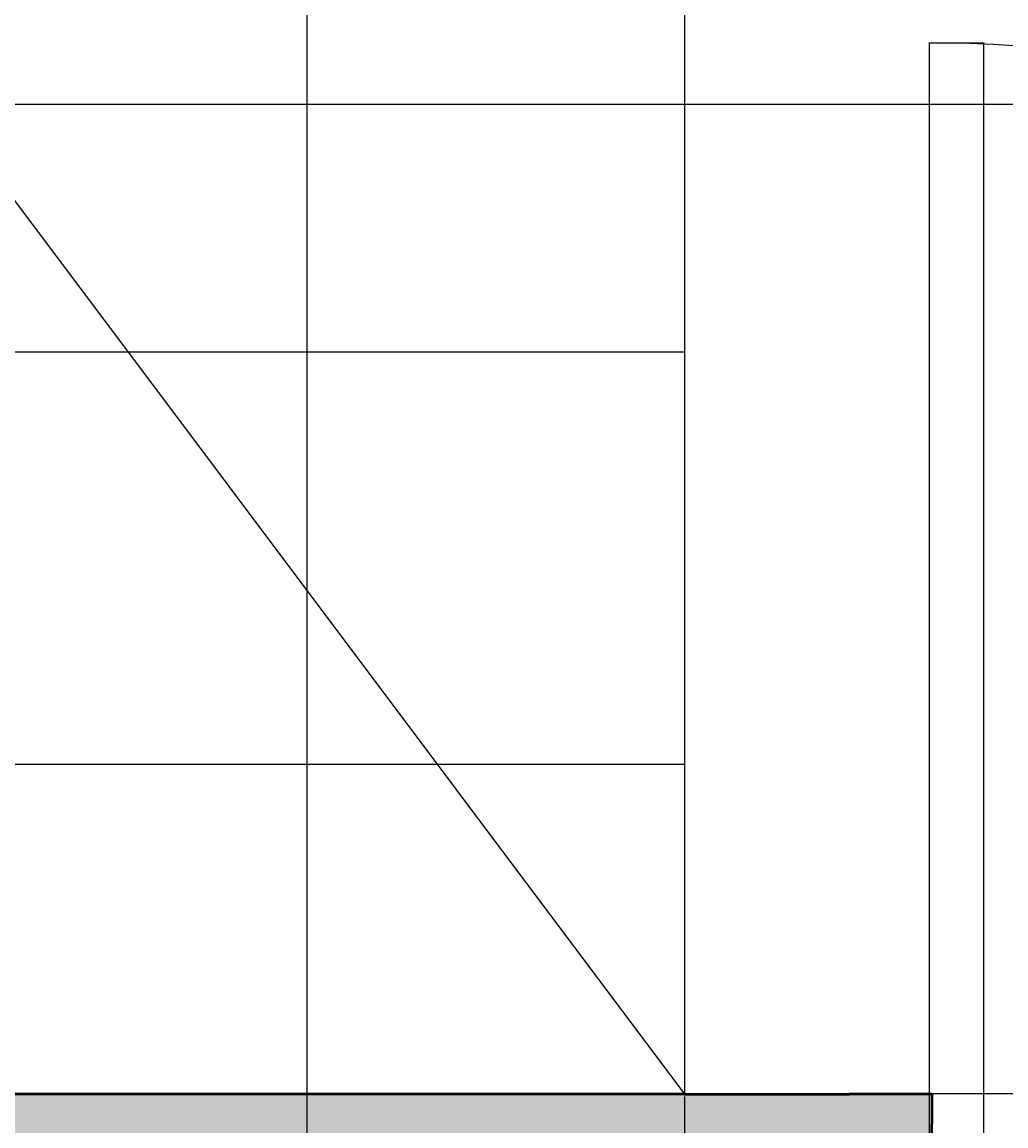
# Model space of a CAD drawing. Units: inches. Extents: x 2231 to 2461, y 2045 to 2455.
# Tile 5 of 95: x 2279 to 2303, y 2072 to 2099. Entities that reach past the tile are written whole.
import ezdxf

# ---------------------------------------------------------------- set-up
doc = ezdxf.new("R2010")
doc.units = ezdxf.units.IN
for name, color, linetype, lineweight in [('A-ANNO-DIMS', 2, 'Continuous', 18), ('A-DOOR', 3, 'Continuous', 25), ('A-FLOR-EVTR', 8, 'Continuous', 25), ('A-WALL', 7, 'Continuous', 50)]:
    doc.layers.add(name, color=color, linetype=linetype, lineweight=lineweight)
doc.layers.add('A-WALL-PATT', color=18, linetype='Continuous', lineweight=13, true_color=0x000000)
doc.styles.get("Standard").update_dxf_attribs({"font": 'arial.ttf'})
doc.dimstyles.get("Standard").update_dxf_attribs({"dimtxt": 0.18, "dimasz": 0.18, "dimexe": 0.18, "dimexo": 0.0625, "dimgap": 0.09, "dimtad": 0, "dimtih": 1, "dimtoh": 1, "dimdec": 4, "dimzin": 0, "dimdsep": 46, "dimtxsty": 'Standard', "dimcen": 0.09, "dimadec": 0, "dimazin": 0, "dimtfac": 1, "dimtdec": 4, "dimtofl": 0, "dimtmove": 0, "dimatfit": 3, "dimfxl": 1, "dimtolj": 1, "dimtzin": 0, "dimarcsym": 0})

# ---------------------------------------------------------------- blocks, each defined once
blk = doc.blocks.new('*U5')
blk.add_lwpolyline([(0, 0), (0, 40), (1.75, 40), (1.75, 0)], close=True)
blk.add_arc((0, 0), 40, 0, 90)
blk = doc.blocks.new('*D44')
at = {"layer": 'A-ANNO-DIMS', "color": 0, "lineweight": -2, "transparency": 16777216}
for p, q in [((2294.794, 2072.77), (2294.794, 2044.803)), ((2300.794, 2072.77), (2300.794, 2044.803)), ((2294.974, 2044.983), (2297.644, 2044.983)), ((2300.614, 2044.983), (2297.943, 2044.983))]:
    blk.add_line(p, q, dxfattribs=at)
at = {"layer": 'A-ANNO-DIMS', "color": 0, "transparency": 16777216}
for points in [[(2294.974, 2045.013), (2294.974, 2044.953), (2294.794, 2044.983)], [(2300.614, 2045.013), (2300.614, 2044.953), (2300.794, 2044.983)]]:
    blk.add_solid(points, dxfattribs=at)
at = {"layer": 'Defpoints', "color": 0, "transparency": 16777216}
for p in [(2294.794, 2072.833), (2300.794, 2072.833), (2300.794, 2044.983)]:
    blk.add_point(p, dxfattribs=at)
at = {"layer": 'A-ANNO-DIMS', "color": 0, "transparency": 16777216, "insert": (2297.794, 2044.983), "char_height": 0.18, "attachment_point": 5}
blk.add_mtext('\\A1;6', dxfattribs=at)
blk = doc.blocks.new('*D51')
at = {"layer": 'A-ANNO-DIMS', "color": 0, "lineweight": -2, "transparency": 16777216}
for p, q in [((2258.794, 2306.77), (2258.794, 2044.803)), ((2330.794, 2306.77), (2330.794, 2044.803)), ((2258.974, 2044.983), (2294.576, 2044.983)), ((2330.614, 2044.983), (2295.011, 2044.983))]:
    blk.add_line(p, q, dxfattribs=at)
at = {"layer": 'A-ANNO-DIMS', "color": 0, "transparency": 16777216}
for points in [[(2258.974, 2045.013), (2258.974, 2044.953), (2258.794, 2044.983)], [(2330.614, 2045.013), (2330.614, 2044.953), (2330.794, 2044.983)]]:
    blk.add_solid(points, dxfattribs=at)
at = {"layer": 'Defpoints', "color": 0, "transparency": 16777216}
for p in [(2258.794, 2306.833), (2330.794, 2306.833), (2330.794, 2044.983)]:
    blk.add_point(p, dxfattribs=at)
at = {"layer": 'A-ANNO-DIMS', "color": 0, "transparency": 16777216, "insert": (2294.794, 2044.983), "char_height": 0.18, "attachment_point": 5}
blk.add_mtext('\\A1;72', dxfattribs=at)
blk = doc.blocks.new('*D65')
at = {"layer": 'A-ANNO-DIMS', "color": 0, "lineweight": -2, "transparency": 16777216}
for p, q in [((2285.635, 2189.285), (2285.635, 2044.803)), ((2340.667, 2189.285), (2340.667, 2044.803)), ((2285.815, 2044.983), (2312.758, 2044.983)), ((2340.487, 2044.983), (2313.545, 2044.983))]:
    blk.add_line(p, q, dxfattribs=at)
at = {"layer": 'A-ANNO-DIMS', "color": 0, "transparency": 16777216}
for points in [[(2285.815, 2045.013), (2285.815, 2044.953), (2285.635, 2044.983)], [(2340.487, 2045.013), (2340.487, 2044.953), (2340.667, 2044.983)]]:
    blk.add_solid(points, dxfattribs=at)
at = {"layer": 'Defpoints', "color": 0, "transparency": 16777216}
for p in [(2285.635, 2189.348), (2340.667, 2189.348), (2340.667, 2044.983)]:
    blk.add_point(p, dxfattribs=at)
at = {"layer": 'A-ANNO-DIMS', "color": 0, "transparency": 16777216, "insert": (2313.151, 2044.983), "char_height": 0.18, "attachment_point": 5}
blk.add_mtext('\\A1;55.03', dxfattribs=at)
blk = doc.blocks.new('*D67')
at = {"layer": 'A-ANNO-DIMS', "color": 0, "lineweight": -2, "transparency": 16777216}
for p, q in [((2348.126, 2096.833), (2230.981, 2096.833)), ((2231.161, 2096.653), (2231.161, 2085.013)), ((2231.161, 2073.013), (2231.161, 2084.652)), ((2348.559, 2072.833), (2230.981, 2072.833))]:
    blk.add_line(p, q, dxfattribs=at)
at = {"layer": 'A-ANNO-DIMS', "color": 0, "transparency": 16777216}
for points in [[(2231.131, 2096.653), (2231.191, 2096.653), (2231.161, 2096.833)], [(2231.131, 2073.013), (2231.191, 2073.013), (2231.161, 2072.833)]]:
    blk.add_solid(points, dxfattribs=at)
at = {"layer": 'Defpoints', "color": 0, "transparency": 16777216}
for p in [(2348.189, 2096.833), (2231.161, 2072.833), (2348.622, 2072.833)]:
    blk.add_point(p, dxfattribs=at)
at = {"layer": 'A-ANNO-DIMS', "color": 0, "transparency": 16777216, "insert": (2231.161, 2084.833), "char_height": 0.18, "attachment_point": 5}
blk.add_mtext('\\A1;24', dxfattribs=at)

msp = doc.modelspace()

# ---------------------------------------------------------------- hatches: boundary and pattern name
at = {"layer": 'A-WALL-PATT'}
h = msp.add_hatch(color=256, dxfattribs=at)
h.dxf.hatch_style = 1
h.paths.add_polyline_path([(2441.7935, 2269.1535), (2432.7935, 2269.1535), (2432.7935, 2186.8328), (2396.7935, 2186.8328), (2396.7935, 2286.8328), (2394.7935, 2286.8328), (2394.7935, 2186.8328), (2334.7935, 2186.8328), (2334.7935, 2182.8328), (2432.7935, 2182.8328), (2432.7935, 2072.8328), (2416.6639, 2072.8328), (2416.6639, 2063.8328), (2441.7935, 2063.8328)])
h.paths.add_polyline_path([(2368.6639, 2072.8328), (2367.04, 2072.8328), (2330.7942, 2072.8328), (2330.7397, 2063.8328), (2368.6639, 2063.8328)])
h.paths.add_polyline_path([(2300.7392, 2068.3328), (2300.7392, 2072.8328), (2298.7935, 2072.8328), (2294.7935, 2072.8328), (2258.7935, 2072.8328), (2258.7935, 2120.8328), (2294.7935, 2120.8328), (2298.7935, 2120.8328), (2298.7935, 2128.8328), (2294.7935, 2128.8328), (2294.7935, 2124.8328), (2258.7935, 2124.8328), (2258.7935, 2182.8328), (2294.7935, 2182.8328), (2294.7935, 2174.8328), (2298.7935, 2174.8328), (2298.7935, 2182.8328), (2304.7935, 2182.8328), (2304.7935, 2186.8328), (2258.7935, 2186.8328), (2258.7935, 2221.999), (2249.7935, 2221.999), (2249.7935, 2063.8328), (2300.7392, 2063.8328)])
h.paths.add_polyline_path([(2391.9338, 2435.8328), (2333.82, 2435.8328), (2333.82, 2426.8328), (2368.7935, 2426.8328), (2368.7935, 2374.9508), (2368.7935, 2370.8328), (2372.3935, 2370.8328), (2372.7935, 2370.8328), (2372.7935, 2426.8328), (2391.9338, 2426.8328)])
h.paths.add_polyline_path([(2441.7935, 2435.8328), (2415.9338, 2435.8328), (2415.9338, 2426.8328), (2432.7935, 2426.8328), (2432.7935, 2334.8328), (2372.7935, 2334.8328), (2372.7935, 2346.8328), (2368.7935, 2346.8328), (2368.7935, 2306.8328), (2360.7935, 2306.8328), (2360.7935, 2302.8328), (2368.7935, 2302.8328), (2372.7935, 2302.8328), (2372.7935, 2330.8328), (2432.7935, 2330.8328), (2432.7935, 2317.1535), (2441.7935, 2317.1535)])
h.paths.add_polyline_path([(2285.82, 2435.8328), (2249.7935, 2435.8328), (2249.7935, 2269.999), (2258.7935, 2269.999), (2258.7935, 2302.8328), (2318.8168, 2302.8328), (2330.7935, 2302.8328), (2330.7935, 2306.8328), (2258.7935, 2306.8328), (2258.7935, 2426.8328), (2285.82, 2426.8328)])

# ---------------------------------------------------------------- linework, layer by layer
at = {"layer": 'A-FLOR-EVTR'}
for p, q in [((2258.7935, 2120.8328), (2294.7935, 2072.8328)), ((2294.7935, 2120.8328), (2294.7935, 2072.8328)), ((2258.7935, 2090.8328), (2294.7935, 2090.8328)), ((2258.7935, 2080.8328), (2294.7935, 2080.8328)), ((2294.7935, 2072.8328), (2258.7935, 2072.8328))]:
    msp.add_line(p, q, dxfattribs=at)
at = {"layer": 'A-WALL'}
for p, q in [((2294.7935, 2072.8328), (2258.7935, 2072.8328)), ((2294.7935, 2072.8328), (2298.7935, 2072.8328)), ((2300.7936, 2072.8328), (2298.7935, 2072.8328)), ((2300.7936, 2072.8328), (2300.739, 2063.7965))]:
    msp.add_line(p, q, dxfattribs=at)

# ---------------------------------------------------------------- block references
at = {"layer": 'A-DOOR', "xscale": 0.75, "yscale": 0.75, "zscale": 0.75}
msp.add_blockref('*U5', (2300.7392, 2068.3328), dxfattribs=at)

# ---------------------------------------------------------------- dimensions: what is measured, and where the dimension line sits
at = {"layer": 'A-ANNO-DIMS'}
for base, p1, p2, override, picture, middle in [((2330.7935, 2044.9825), (2258.7935, 2306.8328), (2330.7935, 2306.8328), {"dimdec": 0, "dimlfac": 1, "dimrnd": 0, "dimzin": 0, "dimdsep": 46, "dimlunit": 2}, '*D51', (2294.7935, 2044.9825)), ((2340.6673, 2044.9825), (2285.6353, 2189.3477), (2340.6673, 2189.3477), {"dimdec": 2, "dimlfac": 1, "dimrnd": 0, "dimzin": 0, "dimdsep": 46, "dimlunit": 2}, '*D65', (2313.1513, 2044.9825)), ((2300.7936, 2044.9825), (2294.7935, 2072.8328), (2300.7936, 2072.8328), {"dimdec": 0, "dimlfac": 1, "dimrnd": 0, "dimzin": 0, "dimdsep": 46, "dimlunit": 2}, '*D44', (2297.7936, 2044.9825))]:
    dim = msp.add_linear_dim(base=base, p1=p1, p2=p2, dimstyle='Standard', override=override, dxfattribs=at)
    dim.commit()
    dim.dimension.update_dxf_attribs({"geometry": picture, "text_midpoint": middle})
dim = msp.add_linear_dim(base=(2231.161, 2072.8328), p1=(2348.1888, 2096.8328), p2=(2348.6219, 2072.8328), angle=90, dimstyle='Standard', override={"dimdec": 0, "dimlfac": 1, "dimrnd": 0, "dimzin": 0, "dimdsep": 46, "dimlunit": 2}, dxfattribs=at)
dim.commit()
dim.dimension.update_dxf_attribs({"geometry": '*D67', "text_midpoint": (2231.161, 2084.8328)})

doc.saveas('drawing.dxf')
